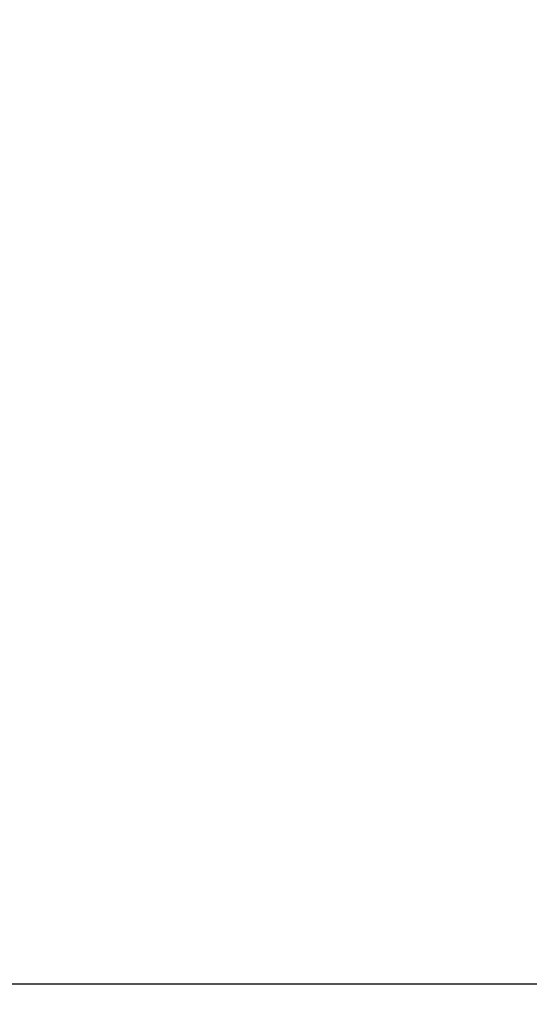
# Model space of a CAD drawing. Units: millimetres. Extents: x 0 to 2267, y 0 to 1823.
# Tile 7 of 256: x 1459 to 1482, y 1116 to 1162. Entities that reach past the tile are written whole.
import ezdxf

# ---------------------------------------------------------------- set-up
doc = ezdxf.new("R2010")
doc.units = ezdxf.units.MM
doc.header["$MEASUREMENT"] = 0
doc.layers.add('M-DIMS', color=2, linetype='Continuous', lineweight=25)
doc.layers.add('M-HATC', color=252, linetype='Continuous', lineweight=18)
doc.styles.get("Standard").update_dxf_attribs({"font": 'arial.ttf'})
doc.dimstyles.get("Standard").update_dxf_attribs({"dimtxt": 7, "dimasz": 4, "dimexe": 0.18, "dimexo": 0.0625, "dimgap": 0.09, "dimtad": 0, "dimdec": 0, "dimzin": 0, "dimdsep": 46, "dimtxsty": 'Standard', "dimcen": 0.09, "dimadec": 0, "dimazin": 0, "dimtfac": 1, "dimtdec": 0, "dimtofl": 0, "dimtmove": 0, "dimatfit": 3, "dimfxl": 1, "dimtolj": 1, "dimtzin": 0, "dimarcsym": 0})

# ---------------------------------------------------------------- blocks, each defined once
blk = doc.blocks.new('*D9')
at = {"layer": 'Defpoints', "color": 0, "transparency": 16777216}
for p in [(1332.087, 1117.417), (1505.929, 1117.417), (1505.929, 1077.417)]:
    blk.add_point(p, dxfattribs=at)
at = {"layer": 'M-DIMS', "color": 0, "lineweight": -2, "transparency": 16777216}
for p, q in [((1505.866, 1117.417), (1331.907, 1117.417)), ((1332.087, 1113.417), (1332.087, 1102.65)), ((1332.087, 1081.417), (1332.087, 1092.184)), ((1505.866, 1077.417), (1331.907, 1077.417))]:
    blk.add_line(p, q, dxfattribs=at)
at = {"layer": 'M-DIMS', "color": 0, "transparency": 16777216}
for points in [[(1331.42, 1113.417), (1332.753, 1113.417), (1332.087, 1117.417)], [(1331.42, 1081.417), (1332.753, 1081.417), (1332.087, 1077.417)]]:
    blk.add_solid(points, dxfattribs=at)
at = {"layer": 'M-DIMS', "color": 0, "transparency": 16777216, "insert": (1332.087, 1097.417), "char_height": 7, "attachment_point": 5, "rotation": 90}
blk.add_mtext('\\A1;40', dxfattribs=at)
blk = doc.blocks.new('*D10')
at = {"layer": 'Defpoints', "color": 0, "transparency": 16777216}
for p in [(1332.087, 1287.766), (1505.929, 1287.766), (1505.929, 1117.417)]:
    blk.add_point(p, dxfattribs=at)
at = {"layer": 'M-DIMS', "color": 0, "lineweight": -2, "transparency": 16777216}
for p, q in [((1505.866, 1287.766), (1331.907, 1287.766)), ((1332.087, 1283.766), (1332.087, 1216.908)), ((1332.087, 1121.417), (1332.087, 1188.275)), ((1505.866, 1117.417), (1331.907, 1117.417))]:
    blk.add_line(p, q, dxfattribs=at)
at = {"layer": 'M-DIMS', "color": 0, "transparency": 16777216}
for points in [[(1331.42, 1283.766), (1332.753, 1283.766), (1332.087, 1287.766)], [(1331.42, 1121.417), (1332.753, 1121.417), (1332.087, 1117.417)]]:
    blk.add_solid(points, dxfattribs=at)
at = {"layer": 'M-DIMS', "color": 0, "transparency": 16777216, "insert": (1332.087, 1202.591), "char_height": 7, "attachment_point": 5, "rotation": 90}
blk.add_mtext('\\A1;170.35', dxfattribs=at)

msp = doc.modelspace()

# ---------------------------------------------------------------- hatches: boundary and pattern name
at = {"layer": 'M-HATC'}
h = msp.add_hatch(color=256, dxfattribs=at)
h.dxf.hatch_style = 1
h.paths.add_polyline_path([(2055.771, 1603.062), (1381.087, 1603.062), (1381.087, 1598.062), (2055.771, 1598.062)])
h.paths.add_polyline_path([(2055.771, 1598.062), (1381.087, 1598.062), (1381.087, 1593.062), (2055.771, 1593.062)])
h.paths.add_polyline_path([(2051.307, 1536.761), (1385.55, 1536.761), (1385.55, 1526.761), (1387.55, 1526.761), (1388.537, 1525.053), (1385.332, 1521.233), (1385.332, 1521.223), (2050.254, 1522.749), (2048.321, 1525.053), (2049.307, 1526.761), (2051.307, 1526.761)])
edge = h.paths.add_edge_path()
edge.add_arc((1847.535, 1379.149), 135, 222.60306, 222.89085, ccw=False)
edge.add_line((1748.166, 1287.766), (1683.092, 1287.766))
edge.add_arc((1583.724, 1379.149), 135, 317.10915, 317.39694, ccw=False)
edge.add_arc((1678.969, 1290.671), 5, 222.8909, 317.1091, ccw=False)
edge.add_arc((1774.213, 1379.149), 135, 222.60306, 222.89085, ccw=False)
edge.add_line((1674.845, 1287.766), (1609.771, 1287.766))
edge.add_arc((1510.403, 1379.149), 135, 317.10915, 317.39694, ccw=False)
edge.add_arc((1605.647, 1290.671), 5, 222.8909, 317.1091, ccw=False)
edge.add_arc((1700.892, 1379.149), 135, 222.60306, 222.89085, ccw=False)
edge.add_line((1601.524, 1287.766), (1536.45, 1287.766))
edge.add_arc((1437.081, 1379.149), 135, 317.10915, 317.39694, ccw=False)
edge.add_arc((1532.326, 1290.671), 5, 222.8909, 317.1091, ccw=False)
edge.add_arc((1627.571, 1379.149), 135, 222.60306, 222.89085, ccw=False)
edge.add_line((1528.203, 1287.766), (1505.929, 1287.766))
edge.add_spline(control_points=[(1505.929, 1287.766), (1504.262, 1287.766), (1504.262, 1282.766), (1505.929, 1282.766)], knot_values=[0, 0, 0, 0, 5, 5, 5, 5], degree=3, periodic=0)
edge.add_line((1505.929, 1282.766), (1930.929, 1282.766))
edge.add_spline(control_points=[(1930.929, 1282.766), (1932.596, 1282.766), (1932.596, 1287.766), (1930.929, 1287.766)], knot_values=[0, 0, 0, 0, 5, 5, 5, 5], degree=3, periodic=0)
edge.add_line((1930.929, 1287.766), (1903.056, 1287.766))
edge.add_arc((1803.688, 1379.149), 135, 317.10915, 317.39694, ccw=False)
edge.add_arc((1898.932, 1290.671), 5, 222.8909, 317.1091, ccw=False)
edge.add_arc((1994.177, 1379.149), 135, 222.60306, 222.89085, ccw=False)
edge.add_line((1894.809, 1287.766), (1829.735, 1287.766))
edge.add_arc((1730.366, 1379.149), 135, 317.10915, 317.39694, ccw=False)
edge.add_arc((1825.611, 1290.671), 5, 222.8909, 317.1091, ccw=False)
edge.add_arc((1920.856, 1379.149), 135, 222.60306, 222.89085, ccw=False)
edge.add_line((1821.487, 1287.766), (1756.413, 1287.766))
edge.add_arc((1657.045, 1379.149), 135, 317.10915, 317.39694, ccw=False)
edge.add_arc((1752.29, 1290.671), 5, 222.8909, 317.1091, ccw=False)
edge = h.paths.add_edge_path()
edge.add_spline(control_points=[(1843.429, 1227.247), (1845.096, 1227.247), (1845.096, 1232.247), (1843.429, 1232.247)], knot_values=[0, 0, 0, 0, 5, 5, 5, 5], degree=3, periodic=0)
edge.add_line((1843.429, 1232.247), (1593.429, 1232.247))
edge.add_spline(control_points=[(1593.429, 1232.247), (1591.762, 1232.247), (1591.762, 1227.247), (1593.429, 1227.247)], knot_values=[0, 0, 0, 0, 5, 5, 5, 5], degree=3, periodic=0)
edge.add_line((1593.429, 1227.247), (1843.429, 1227.247))
h.paths.add_polyline_path([(1905.929, 1127.417), (1530.929, 1127.417, 0.414214), (1520.929, 1117.417), (1530.929, 1117.417), (1915.929, 1117.417, 0.414214)])
edge = h.paths.add_edge_path()
edge.add_arc((1397.086, 1498.408), 12.73, 90.7821, 190.8787, ccw=False)
edge.add_line((1396.912, 1511.136), (1428.01, 1511.349))
edge.add_line((1428.01, 1511.349), (1433.01, 1511.349))
edge.add_line((1433.01, 1511.349), (1434.439, 1511.349))
edge.add_arc((1419.474, 1498.08), 20, 41.561, 74.0821)
edge.add_line((1424.959, 1517.314), (1399.935, 1517.256))
edge.add_spline(control_points=[(1399.931, 1517.256), (1399.884, 1517.213), (1399.833, 1517.169), (1399.777, 1517.124)], knot_values=[11.567499, 11.567499, 11.567499, 11.567499, 11.814249, 11.814249, 11.814249, 11.814249], degree=3, periodic=0)
edge.add_spline(control_points=[(1399.633, 1517.01), (1399.583, 1516.972), (1399.531, 1516.934), (1399.476, 1516.895)], knot_values=[11.167718, 11.167718, 11.167718, 11.167718, 11.365188, 11.365188, 11.365188, 11.365188], degree=3, periodic=0)
edge.add_spline(control_points=[(1399.34, 1516.8), (1399.151, 1516.672), (1398.938, 1516.538), (1398.704, 1516.399)], knot_values=[10.376405, 10.376405, 10.376405, 10.376405, 11.00994, 11.00994, 11.00994, 11.00994], degree=3, periodic=0)
edge.add_spline(control_points=[(1398.657, 1516.372), (1398.579, 1516.326), (1398.498, 1516.28), (1398.415, 1516.233)], knot_values=[10.125175, 10.125175, 10.125175, 10.125175, 10.334406, 10.334406, 10.334406, 10.334406], degree=3, periodic=0)
edge.add_spline(control_points=[(1398.264, 1516.149), (1398.196, 1516.111), (1398.126, 1516.073), (1398.055, 1516.035)], knot_values=[9.832246, 9.832246, 9.832246, 9.832246, 9.999658, 9.999658, 9.999658, 9.999658], degree=3, periodic=0)
edge.add_spline(control_points=[(1397.999, 1516.005), (1397.731, 1515.862), (1397.446, 1515.717), (1397.147, 1515.571)], knot_values=[9.161808, 9.161808, 9.161808, 9.161808, 9.787769, 9.787769, 9.787769, 9.787769], degree=3, periodic=0)
edge.add_spline(control_points=[(1397.147, 1515.571), (1396.842, 1515.423), (1396.522, 1515.274), (1396.191, 1515.126)], knot_values=[8.524455, 8.524455, 8.524455, 8.524455, 9.161808, 9.161808, 9.161808, 9.161808], degree=3, periodic=0)
edge.add_spline(control_points=[(1396.078, 1515.076), (1395.985, 1515.035), (1395.892, 1514.994), (1395.798, 1514.953)], knot_values=[8.275193, 8.275193, 8.275193, 8.275193, 8.451726, 8.451726, 8.451726, 8.451726], degree=3, periodic=0)
edge.add_spline(control_points=[(1395.602, 1514.869), (1395.5, 1514.826), (1395.397, 1514.782), (1395.293, 1514.739)], knot_values=[7.962917, 7.962917, 7.962917, 7.962917, 8.152764, 8.152764, 8.152764, 8.152764], degree=3, periodic=0)
edge.add_spline(control_points=[(1395.212, 1514.706), (1394.828, 1514.547), (1394.435, 1514.393), (1394.036, 1514.244)], knot_values=[7.21254, 7.21254, 7.21254, 7.21254, 7.913148, 7.913148, 7.913148, 7.913148], degree=3, periodic=0)
edge.add_spline(control_points=[(1394.036, 1514.244), (1393.708, 1514.121), (1393.375, 1514.003), (1393.043, 1513.889)], knot_values=[6.633733, 6.633733, 6.633733, 6.633733, 7.21254, 7.21254, 7.21254, 7.21254], degree=3, periodic=0)
edge.add_spline(control_points=[(1392.821, 1513.815), (1392.72, 1513.781), (1392.618, 1513.748), (1392.517, 1513.715)], knot_values=[6.328796, 6.328796, 6.328796, 6.328796, 6.505493, 6.505493, 6.505493, 6.505493], degree=3, periodic=0)
edge.add_spline(control_points=[(1392.517, 1513.715), (1392.319, 1513.652), (1392.121, 1513.59), (1391.924, 1513.531)], knot_values=[5.984605, 5.984605, 5.984605, 5.984605, 6.328796, 6.328796, 6.328796, 6.328796], degree=3, periodic=0)
edge.add_spline(control_points=[(1391.792, 1513.491), (1391.312, 1513.35), (1390.838, 1513.224), (1390.378, 1513.117)], knot_values=[5.066697, 5.066697, 5.066697, 5.066697, 5.907055, 5.907055, 5.907055, 5.907055], degree=3, periodic=0)
edge.add_spline(control_points=[(1390.378, 1513.117), (1390.18, 1513.071), (1389.984, 1513.028), (1389.791, 1512.99)], knot_values=[4.70367, 4.70367, 4.70367, 4.70367, 5.066695, 5.066695, 5.066695, 5.066695], degree=3, periodic=0)
edge.add_spline(control_points=[(1389.422, 1512.92), (1389.246, 1512.889), (1389.073, 1512.862), (1388.904, 1512.838)], knot_values=[4.130571, 4.130571, 4.130571, 4.130571, 4.469816, 4.469816, 4.469816, 4.469816], degree=3, periodic=0)
edge.add_spline(control_points=[(1388.904, 1512.838), (1388.591, 1512.795), (1388.291, 1512.764), (1388.007, 1512.749)], knot_values=[3.504031, 3.504031, 3.504031, 3.504031, 4.130571, 4.130571, 4.130571, 4.130571], degree=3, periodic=0)
edge.add_spline(control_points=[(1387.936, 1512.746), (1387.854, 1512.742), (1387.773, 1512.74), (1387.694, 1512.739)], knot_values=[3.268866, 3.268866, 3.268866, 3.268866, 3.451164, 3.451164, 3.451164, 3.451164], degree=3, periodic=0)
edge.add_spline(control_points=[(1387.335, 1512.744), (1387.208, 1512.75), (1387.085, 1512.76), (1386.967, 1512.774)], knot_values=[2.670686, 2.670686, 2.670686, 2.670686, 2.984, 2.984, 2.984, 2.984], degree=3, periodic=0)
edge.add_spline(control_points=[(1386.833, 1512.792), (1386.821, 1512.794), (1386.809, 1512.796), (1386.797, 1512.798)], knot_values=[2.516981, 2.516981, 2.516981, 2.516981, 2.549528, 2.549528, 2.549528, 2.549528], degree=3, periodic=0)
edge.add_spline(control_points=[(1386.453, 1512.873), (1386.426, 1512.881), (1386.399, 1512.889), (1386.373, 1512.897)], knot_values=[2.095869, 2.095869, 2.095869, 2.095869, 2.17941, 2.17941, 2.17941, 2.17941], degree=3, periodic=0)
edge.add_spline(control_points=[(1386.069, 1513.019), (1386.063, 1513.022), (1386.058, 1513.025), (1386.052, 1513.028)], knot_values=[1.72453, 1.72453, 1.72453, 1.72453, 1.745933, 1.745933, 1.745933, 1.745933], degree=3, periodic=0)
edge.add_arc((1399.474, 1498.08), 20, 131.8243, 180)
edge.add_arc((1630.334, 1505.548), 250.971, 181.70518, 236.42798)
edge.add_arc((1605.34, 1483.304), 218.782, 238.66083, 243.34961)
edge.add_arc((1647.091, 1510.359), 262.899, 183.12984, 237.85344, ccw=False)
h.paths.add_polyline_path([(1406.537, 1391.964, 0.149382), (1491.551, 1296.442, -0.129517)], flags=17)
edge = h.paths.add_edge_path()
edge.add_arc((2037.384, 1498.08), 20, 0, 48.2659)
edge.add_spline(control_points=[(2050.697, 1513.005), (2050.651, 1512.985), (2050.603, 1512.966), (2050.554, 1512.948)], knot_values=[1.835652, 1.835652, 1.835652, 1.835652, 2.000781, 2.000781, 2.000781, 2.000781], degree=3, periodic=0)
edge.add_spline(control_points=[(2050.462, 1512.917), (2050.479, 1512.922), (2050.496, 1512.928), (2050.513, 1512.934)], knot_values=[2.045477, 2.045477, 2.045477, 2.045477, 2.101389, 2.101389, 2.101389, 2.101389], degree=3, periodic=0)
edge.add_spline(control_points=[(2050.129, 1512.834), (2050.198, 1512.847), (2050.266, 1512.862), (2050.331, 1512.879)], knot_values=[2.237629, 2.237629, 2.237629, 2.237629, 2.435841, 2.435841, 2.435841, 2.435841], degree=3, periodic=0)
edge.add_spline(control_points=[(2050.095, 1512.828), (2050.106, 1512.83), (2050.118, 1512.832), (2050.129, 1512.834)], knot_values=[2.435841, 2.435841, 2.435841, 2.435841, 2.468321, 2.468321, 2.468321, 2.468321], degree=3, periodic=0)
edge.add_spline(control_points=[(2049.784, 1512.785), (2049.855, 1512.792), (2049.924, 1512.801), (2049.992, 1512.811)], knot_values=[2.563852, 2.563852, 2.563852, 2.563852, 2.748541, 2.748541, 2.748541, 2.748541], degree=3, periodic=0)
edge.add_spline(control_points=[(2049.405, 1512.762), (2049.536, 1512.765), (2049.663, 1512.773), (2049.784, 1512.785)], knot_values=[2.748541, 2.748541, 2.748541, 2.748541, 3.064882, 3.064882, 3.064882, 3.064882], degree=3, periodic=0)
edge.add_spline(control_points=[(2049.17, 1512.76), (2049.234, 1512.759), (2049.297, 1512.759), (2049.358, 1512.761)], knot_values=[3.102309, 3.102309, 3.102309, 3.102309, 3.2503, 3.2503, 3.2503, 3.2503], degree=3, periodic=0)
edge.add_spline(control_points=[(2048.857, 1512.769), (2048.964, 1512.764), (2049.068, 1512.761), (2049.17, 1512.76)], knot_values=[3.2503, 3.2503, 3.2503, 3.2503, 3.486069, 3.486069, 3.486069, 3.486069], degree=3, periodic=0)
edge.add_spline(control_points=[(2048.692, 1512.779), (2048.373, 1512.801), (2048.035, 1512.841), (2047.682, 1512.897)], knot_values=[3.606429, 3.606429, 3.606429, 3.606429, 4.2989, 4.2989, 4.2989, 4.2989], degree=3, periodic=0)
edge.add_spline(control_points=[(2047.682, 1512.897), (2047.546, 1512.919), (2047.408, 1512.942), (2047.268, 1512.969)], knot_values=[4.2989, 4.2989, 4.2989, 4.2989, 4.565769, 4.565769, 4.565769, 4.565769], degree=3, periodic=0)
edge.add_spline(control_points=[(2047.268, 1512.969), (2047.145, 1512.991), (2047.021, 1513.016), (2046.895, 1513.042)], knot_values=[4.565769, 4.565769, 4.565769, 4.565769, 4.799971, 4.799971, 4.799971, 4.799971], degree=3, periodic=0)
edge.add_spline(control_points=[(2046.895, 1513.042), (2046.529, 1513.119), (2046.151, 1513.209), (2045.768, 1513.311)], knot_values=[4.799971, 4.799971, 4.799971, 4.799971, 5.483718, 5.483718, 5.483718, 5.483718], degree=3, periodic=0)
edge.add_spline(control_points=[(2045.768, 1513.311), (2045.372, 1513.415), (2044.97, 1513.532), (2044.566, 1513.659)], knot_values=[5.483718, 5.483718, 5.483718, 5.483718, 6.187866, 6.187866, 6.187866, 6.187866], degree=3, periodic=0)
edge.add_spline(control_points=[(2044.566, 1513.659), (2044.415, 1513.706), (2044.263, 1513.755), (2044.112, 1513.805)], knot_values=[6.187866, 6.187866, 6.187866, 6.187866, 6.451551, 6.451551, 6.451551, 6.451551], degree=3, periodic=0)
edge.add_spline(control_points=[(2044.112, 1513.805), (2043.997, 1513.843), (2043.882, 1513.881), (2043.767, 1513.92)], knot_values=[6.451551, 6.451551, 6.451551, 6.451551, 6.651434, 6.651434, 6.651434, 6.651434], degree=3, periodic=0)
edge.add_spline(control_points=[(2043.767, 1513.92), (2043.372, 1514.055), (2042.977, 1514.198), (2042.589, 1514.346)], knot_values=[6.651434, 6.651434, 6.651434, 6.651434, 7.338879, 7.338879, 7.338879, 7.338879], degree=3, periodic=0)
edge.add_spline(control_points=[(2042.589, 1514.346), (2042.164, 1514.507), (2041.746, 1514.675), (2041.341, 1514.846)], knot_values=[7.338879, 7.338879, 7.338879, 7.338879, 8.089209, 8.089209, 8.089209, 8.089209], degree=3, periodic=0)
edge.add_spline(control_points=[(2041.341, 1514.846), (2041.103, 1514.946), (2040.869, 1515.048), (2040.64, 1515.15)], knot_values=[8.089209, 8.089209, 8.089209, 8.089209, 8.529587, 8.529587, 8.529587, 8.529587], degree=3, periodic=0)
edge.add_spline(control_points=[(2040.51, 1515.209), (2040.082, 1515.402), (2039.675, 1515.597), (2039.295, 1515.789)], knot_values=[8.613818, 8.613818, 8.613818, 8.613818, 9.44571, 9.44571, 9.44571, 9.44571], degree=3, periodic=0)
edge.add_spline(control_points=[(2039.295, 1515.789), (2039.062, 1515.907), (2038.839, 1516.025), (2038.629, 1516.14)], knot_values=[9.44571, 9.44571, 9.44571, 9.44571, 9.956404, 9.956404, 9.956404, 9.956404], degree=3, periodic=0)
edge.add_spline(control_points=[(2038.629, 1516.14), (2038.519, 1516.2), (2038.412, 1516.26), (2038.309, 1516.319)], knot_values=[9.956404, 9.956404, 9.956404, 9.956404, 10.223542, 10.223542, 10.223542, 10.223542], degree=3, periodic=0)
edge.add_spline(control_points=[(2038.309, 1516.319), (2038.214, 1516.374), (2038.122, 1516.428), (2038.033, 1516.481)], knot_values=[10.223542, 10.223542, 10.223542, 10.223542, 10.47051, 10.47051, 10.47051, 10.47051], degree=3, periodic=0)
edge.add_spline(control_points=[(2038.033, 1516.481), (2037.786, 1516.63), (2037.564, 1516.773), (2037.372, 1516.909)], knot_values=[10.47051, 10.47051, 10.47051, 10.47051, 11.15767, 11.15767, 11.15767, 11.15767], degree=3, periodic=0)
edge.add_spline(control_points=[(2037.372, 1516.909), (2037.279, 1516.975), (2037.193, 1517.04), (2037.114, 1517.102)], knot_values=[11.15767, 11.15767, 11.15767, 11.15767, 11.49227, 11.49227, 11.49227, 11.49227], degree=3, periodic=0)
edge.add_spline(control_points=[(2036.856, 1517.326), (2036.915, 1517.269), (2036.981, 1517.21), (2037.056, 1517.149)], knot_values=[11.577341, 11.577341, 11.577341, 11.577341, 11.91035, 11.91035, 11.91035, 11.91035], degree=3, periodic=0)
edge.add_spline(control_points=[(2036.807, 1517.375), (2036.823, 1517.359), (2036.839, 1517.342), (2036.856, 1517.326)], knot_values=[11.91035, 11.91035, 11.91035, 11.91035, 12.007402, 12.007402, 12.007402, 12.007402], degree=3, periodic=0)
edge.add_spline(control_points=[(2036.702, 1517.494), (2036.71, 1517.483), (2036.72, 1517.472), (2036.729, 1517.461)], knot_values=[12.184155, 12.184155, 12.184155, 12.184155, 12.255409, 12.255409, 12.255409, 12.255409], degree=3, periodic=0)
edge.add_spline(control_points=[(2036.616, 1517.621), (2036.62, 1517.613), (2036.624, 1517.606), (2036.629, 1517.598)], knot_values=[12.487913, 12.487913, 12.487913, 12.487913, 12.541035, 12.541035, 12.541035, 12.541035], degree=3, periodic=0)
edge.add_spline(control_points=[(2036.563, 1517.786), (2036.564, 1517.779), (2036.564, 1517.773), (2036.565, 1517.766)], knot_values=[12.911761, 12.911761, 12.911761, 12.911761, 12.968286, 12.968286, 12.968286, 12.968286], degree=3, periodic=0)
edge.add_spline(control_points=[(2036.617, 1517.93), (2036.612, 1517.926), (2036.609, 1517.921), (2036.605, 1517.916)], knot_values=[13.382527, 13.382527, 13.382527, 13.382527, 13.433791, 13.433791, 13.433791, 13.433791], degree=3, periodic=0)
edge.add_spline(control_points=[(2036.749, 1518.017), (2036.736, 1518.012), (2036.724, 1518.006), (2036.712, 1518)], knot_values=[13.726299, 13.726299, 13.726299, 13.726299, 13.809928, 13.809928, 13.809928, 13.809928], degree=3, periodic=0)
edge.add_spline(control_points=[(2036.86, 1518.053), (2036.839, 1518.047), (2036.818, 1518.042), (2036.799, 1518.035)], knot_values=[13.910887, 13.910887, 13.910887, 13.910887, 14.02153, 14.02153, 14.02153, 14.02153], degree=3, periodic=0)
edge.add_line((2036.964, 1518.08), (2032.384, 1518.08))
edge.add_line((2032.384, 1518.08), (2027.384, 1518.08))
edge.add_line((2027.384, 1518.08), (2022.384, 1518.08))
edge.add_line((2022.384, 1518.08), (2017.384, 1518.08))
edge.add_arc((2017.384, 1498.08), 20, 90, 138.439)
edge.add_line((2002.419, 1511.349), (2003.848, 1511.349))
edge.add_line((2003.848, 1511.349), (2008.848, 1511.349))
edge.add_line((2008.848, 1511.349), (2039.772, 1511.138))
edge.add_arc((2039.772, 1498.408), 12.73, -10.8787, 90, ccw=False)
edge.add_arc((1789.767, 1510.359), 262.899, 302.14656, 356.87016, ccw=False)
edge.add_arc((1831.518, 1483.304), 218.782, 296.65039, 301.33917)
edge.add_arc((1806.524, 1505.548), 250.971, 303.57202, 358.29482)
h.paths.add_polyline_path([(2030.321, 1391.964, -0.129517), (1945.307, 1296.442, 0.149382)], flags=17)
edge = h.paths.add_edge_path()
edge.add_spline(control_points=[(2037.246, 1518.082), (2037.29, 1518.081), (2037.336, 1518.08), (2037.384, 1518.08)], knot_values=[0.000012, 0.000012, 0.000012, 0.000012, 0.144754, 0.144754, 0.144754, 0.144754], degree=3, periodic=0)
edge.add_line((2037.336, 1518.08), (2037.01, 1518.08))
edge.add_spline(control_points=[(2037.01, 1518.08), (2036.982, 1518.077), (2036.956, 1518.073), (2036.931, 1518.068)], knot_values=[14.13465, 14.13465, 14.13465, 14.13465, 14.247197, 14.247197, 14.247197, 14.247197], degree=3, periodic=0)
edge.add_spline(control_points=[(2036.931, 1518.068), (2036.928, 1518.067), (2036.924, 1518.067), (2036.921, 1518.066)], knot_values=[14.118315, 14.118315, 14.118315, 14.118315, 14.13465, 14.13465, 14.13465, 14.13465], degree=3, periodic=0)
edge.add_spline(control_points=[(2036.921, 1518.066), (2036.912, 1518.064), (2036.903, 1518.063), (2036.895, 1518.061)], knot_values=[14.078086, 14.078086, 14.078086, 14.078086, 14.118315, 14.118315, 14.118315, 14.118315], degree=3, periodic=0)
edge.add_spline(control_points=[(2036.895, 1518.061), (2036.883, 1518.058), (2036.872, 1518.056), (2036.86, 1518.053)], knot_values=[14.02153, 14.02153, 14.02153, 14.02153, 14.078086, 14.078086, 14.078086, 14.078086], degree=3, periodic=0)
edge.add_spline(control_points=[(2036.86, 1518.053), (2036.839, 1518.047), (2036.818, 1518.042), (2036.799, 1518.035)], knot_values=[13.910887, 13.910887, 13.910887, 13.910887, 14.02153, 14.02153, 14.02153, 14.02153], degree=3, periodic=0)
edge.add_spline(control_points=[(2036.799, 1518.035), (2036.798, 1518.035), (2036.797, 1518.035), (2036.797, 1518.035)], knot_values=[13.906906, 13.906906, 13.906906, 13.906906, 13.910887, 13.910887, 13.910887, 13.910887], degree=3, periodic=0)
edge.add_spline(control_points=[(2036.797, 1518.035), (2036.788, 1518.032), (2036.78, 1518.029), (2036.772, 1518.026)], knot_values=[13.857826, 13.857826, 13.857826, 13.857826, 13.906906, 13.906906, 13.906906, 13.906906], degree=3, periodic=0)
edge.add_spline(control_points=[(2036.772, 1518.026), (2036.764, 1518.023), (2036.756, 1518.02), (2036.749, 1518.017)], knot_values=[13.809928, 13.809928, 13.809928, 13.809928, 13.857826, 13.857826, 13.857826, 13.857826], degree=3, periodic=0)
edge.add_spline(control_points=[(2036.749, 1518.017), (2036.736, 1518.012), (2036.724, 1518.006), (2036.712, 1518)], knot_values=[13.726299, 13.726299, 13.726299, 13.726299, 13.809928, 13.809928, 13.809928, 13.809928], degree=3, periodic=0)
edge.add_spline(control_points=[(2036.712, 1518), (2036.712, 1518), (2036.712, 1518), (2036.711, 1518)], knot_values=[13.723993, 13.723993, 13.723993, 13.723993, 13.726299, 13.726299, 13.726299, 13.726299], degree=3, periodic=0)
edge.add_spline(control_points=[(2036.711, 1518), (2036.706, 1517.997), (2036.701, 1517.994), (2036.696, 1517.992)], knot_values=[13.686536, 13.686536, 13.686536, 13.686536, 13.723993, 13.723993, 13.723993, 13.723993], degree=3, periodic=0)
edge.add_spline(control_points=[(2036.696, 1517.992), (2036.692, 1517.989), (2036.687, 1517.987), (2036.683, 1517.984)], knot_values=[13.651251, 13.651251, 13.651251, 13.651251, 13.686536, 13.686536, 13.686536, 13.686536], degree=3, periodic=0)
edge.add_spline(control_points=[(2036.683, 1517.984), (2036.676, 1517.98), (2036.67, 1517.976), (2036.664, 1517.971)], knot_values=[13.596804, 13.596804, 13.596804, 13.596804, 13.651251, 13.651251, 13.651251, 13.651251], degree=3, periodic=0)
edge.add_spline(control_points=[(2036.664, 1517.971), (2036.664, 1517.971), (2036.663, 1517.971), (2036.663, 1517.971)], knot_values=[13.593956, 13.593956, 13.593956, 13.593956, 13.596804, 13.596804, 13.596804, 13.596804], degree=3, periodic=0)
edge.add_spline(control_points=[(2036.663, 1517.971), (2036.66, 1517.969), (2036.658, 1517.967), (2036.655, 1517.965)], knot_values=[13.570322, 13.570322, 13.570322, 13.570322, 13.593956, 13.593956, 13.593956, 13.593956], degree=3, periodic=0)
edge.add_spline(control_points=[(2036.655, 1517.965), (2036.653, 1517.963), (2036.65, 1517.961), (2036.647, 1517.959)], knot_values=[13.545477, 13.545477, 13.545477, 13.545477, 13.570322, 13.570322, 13.570322, 13.570322], degree=3, periodic=0)
edge.add_spline(control_points=[(2036.647, 1517.959), (2036.647, 1517.959), (2036.647, 1517.959), (2036.647, 1517.959)], knot_values=[13.543931, 13.543931, 13.543931, 13.543931, 13.545477, 13.545477, 13.545477, 13.545477], degree=3, periodic=0)
edge.add_spline(control_points=[(2036.647, 1517.959), (2036.641, 1517.954), (2036.636, 1517.949), (2036.631, 1517.945)], knot_values=[13.488237, 13.488237, 13.488237, 13.488237, 13.543931, 13.543931, 13.543931, 13.543931], degree=3, periodic=0)
edge.add_spline(control_points=[(2036.631, 1517.945), (2036.628, 1517.942), (2036.626, 1517.94), (2036.623, 1517.937)], knot_values=[13.460307, 13.460307, 13.460307, 13.460307, 13.488237, 13.488237, 13.488237, 13.488237], degree=3, periodic=0)
edge.add_spline(control_points=[(2036.623, 1517.937), (2036.622, 1517.936), (2036.62, 1517.934), (2036.618, 1517.932)], knot_values=[13.439712, 13.439712, 13.439712, 13.439712, 13.460307, 13.460307, 13.460307, 13.460307], degree=3, periodic=0)
edge.add_spline(control_points=[(2036.618, 1517.932), (2036.618, 1517.931), (2036.617, 1517.931), (2036.617, 1517.93)], knot_values=[13.433791, 13.433791, 13.433791, 13.433791, 13.439712, 13.439712, 13.439712, 13.439712], degree=3, periodic=0)
edge.add_spline(control_points=[(2036.617, 1517.93), (2036.612, 1517.926), (2036.609, 1517.921), (2036.605, 1517.916)], knot_values=[13.382527, 13.382527, 13.382527, 13.382527, 13.433791, 13.433791, 13.433791, 13.433791], degree=3, periodic=0)
edge.add_spline(control_points=[(2036.605, 1517.916), (2036.603, 1517.913), (2036.6, 1517.91), (2036.598, 1517.907)], knot_values=[13.350017, 13.350017, 13.350017, 13.350017, 13.382527, 13.382527, 13.382527, 13.382527], degree=3, periodic=0)
edge.add_spline(control_points=[(2036.598, 1517.907), (2036.597, 1517.906), (2036.596, 1517.904), (2036.595, 1517.903)], knot_values=[13.333922, 13.333922, 13.333922, 13.333922, 13.350017, 13.350017, 13.350017, 13.350017], degree=3, periodic=0)
edge.add_spline(control_points=[(2036.595, 1517.903), (2036.595, 1517.902), (2036.594, 1517.901), (2036.593, 1517.9)], knot_values=[13.323828, 13.323828, 13.323828, 13.323828, 13.333922, 13.333922, 13.333922, 13.333922], degree=3, periodic=0)
edge.add_spline(control_points=[(2036.593, 1517.9), (2036.59, 1517.895), (2036.588, 1517.891), (2036.585, 1517.886)], knot_values=[13.277545, 13.277545, 13.277545, 13.277545, 13.323828, 13.323828, 13.323828, 13.323828], degree=3, periodic=0)
edge.add_spline(control_points=[(2036.585, 1517.886), (2036.584, 1517.883), (2036.582, 1517.879), (2036.58, 1517.875)], knot_values=[13.240119, 13.240119, 13.240119, 13.240119, 13.277545, 13.277545, 13.277545, 13.277545], degree=3, periodic=0)
edge.add_spline(control_points=[(2036.58, 1517.875), (2036.58, 1517.874), (2036.579, 1517.873), (2036.578, 1517.872)], knot_values=[13.228211, 13.228211, 13.228211, 13.228211, 13.240119, 13.240119, 13.240119, 13.240119], degree=3, periodic=0)
edge.add_spline(control_points=[(2036.578, 1517.872), (2036.578, 1517.87), (2036.577, 1517.869), (2036.577, 1517.868)], knot_values=[13.215717, 13.215717, 13.215717, 13.215717, 13.228211, 13.228211, 13.228211, 13.228211], degree=3, periodic=0)
edge.add_spline(control_points=[(2036.577, 1517.868), (2036.575, 1517.864), (2036.574, 1517.86), (2036.573, 1517.857)], knot_values=[13.179847, 13.179847, 13.179847, 13.179847, 13.215717, 13.215717, 13.215717, 13.215717], degree=3, periodic=0)
edge.add_spline(control_points=[(2036.573, 1517.857), (2036.571, 1517.851), (2036.57, 1517.846), (2036.569, 1517.841)], knot_values=[13.132017, 13.132017, 13.132017, 13.132017, 13.179847, 13.179847, 13.179847, 13.179847], degree=3, periodic=0)
edge.add_spline(control_points=[(2036.569, 1517.841), (2036.568, 1517.84), (2036.568, 1517.839), (2036.568, 1517.838)], knot_values=[13.122482, 13.122482, 13.122482, 13.122482, 13.132017, 13.132017, 13.132017, 13.132017], degree=3, periodic=0)
edge.add_spline(control_points=[(2036.568, 1517.838), (2036.568, 1517.836), (2036.567, 1517.835), (2036.567, 1517.833)], knot_values=[13.105592, 13.105592, 13.105592, 13.105592, 13.122482, 13.122482, 13.122482, 13.122482], degree=3, periodic=0)
edge.add_spline(control_points=[(2036.567, 1517.833), (2036.566, 1517.829), (2036.566, 1517.826), (2036.565, 1517.822)], knot_values=[13.074063, 13.074063, 13.074063, 13.074063, 13.105592, 13.105592, 13.105592, 13.105592], degree=3, periodic=0)
edge.add_spline(control_points=[(2036.565, 1517.822), (2036.565, 1517.822), (2036.565, 1517.822), (2036.565, 1517.822)], knot_values=[13.074043, 13.074043, 13.074043, 13.074043, 13.074063, 13.074063, 13.074063, 13.074063], degree=3, periodic=0)
edge.add_spline(control_points=[(2036.565, 1517.822), (2036.564, 1517.816), (2036.564, 1517.811), (2036.564, 1517.805)], knot_values=[13.021884, 13.021884, 13.021884, 13.021884, 13.074043, 13.074043, 13.074043, 13.074043], degree=3, periodic=0)
edge.add_spline(control_points=[(2036.564, 1517.805), (2036.564, 1517.804), (2036.564, 1517.803), (2036.564, 1517.803)], knot_values=[13.01674, 13.01674, 13.01674, 13.01674, 13.021884, 13.021884, 13.021884, 13.021884], degree=3, periodic=0)
edge.add_spline(control_points=[(2036.564, 1517.803), (2036.563, 1517.801), (2036.563, 1517.798), (2036.563, 1517.796)], knot_values=[12.996438, 12.996438, 12.996438, 12.996438, 13.01674, 13.01674, 13.01674, 13.01674], degree=3, periodic=0)
edge.add_spline(control_points=[(2036.563, 1517.796), (2036.563, 1517.793), (2036.563, 1517.789), (2036.563, 1517.786)], knot_values=[12.968286, 12.968286, 12.968286, 12.968286, 12.996438, 12.996438, 12.996438, 12.996438], degree=3, periodic=0)
edge.add_spline(control_points=[(2036.563, 1517.786), (2036.564, 1517.779), (2036.564, 1517.773), (2036.565, 1517.766)], knot_values=[12.911761, 12.911761, 12.911761, 12.911761, 12.968286, 12.968286, 12.968286, 12.968286], degree=3, periodic=0)
edge.add_spline(control_points=[(2036.565, 1517.766), (2036.565, 1517.766), (2036.565, 1517.766), (2036.565, 1517.766)], knot_values=[12.911017, 12.911017, 12.911017, 12.911017, 12.911761, 12.911761, 12.911761, 12.911761], degree=3, periodic=0)
edge.add_spline(control_points=[(2036.565, 1517.766), (2036.565, 1517.762), (2036.566, 1517.759), (2036.566, 1517.756)], knot_values=[12.88528, 12.88528, 12.88528, 12.88528, 12.911017, 12.911017, 12.911017, 12.911017], degree=3, periodic=0)
edge.add_spline(control_points=[(2036.566, 1517.756), (2036.567, 1517.753), (2036.567, 1517.751), (2036.568, 1517.748)], knot_values=[12.862519, 12.862519, 12.862519, 12.862519, 12.88528, 12.88528, 12.88528, 12.88528], degree=3, periodic=0)
edge.add_spline(control_points=[(2036.568, 1517.748), (2036.568, 1517.747), (2036.568, 1517.747), (2036.568, 1517.746)], knot_values=[12.858885, 12.858885, 12.858885, 12.858885, 12.862519, 12.862519, 12.862519, 12.862519], degree=3, periodic=0)
edge.add_spline(control_points=[(2036.568, 1517.746), (2036.569, 1517.74), (2036.571, 1517.733), (2036.572, 1517.726)], knot_values=[12.8053, 12.8053, 12.8053, 12.8053, 12.858885, 12.858885, 12.858885, 12.858885], degree=3, periodic=0)
edge.add_spline(control_points=[(2036.572, 1517.726), (2036.573, 1517.723), (2036.574, 1517.719), (2036.576, 1517.715)], knot_values=[12.775176, 12.775176, 12.775176, 12.775176, 12.8053, 12.8053, 12.8053, 12.8053], degree=3, periodic=0)
edge.add_spline(control_points=[(2036.576, 1517.715), (2036.576, 1517.713), (2036.577, 1517.71), (2036.578, 1517.708)], knot_values=[12.756759, 12.756759, 12.756759, 12.756759, 12.775176, 12.775176, 12.775176, 12.775176], degree=3, periodic=0)
edge.add_spline(control_points=[(2036.578, 1517.708), (2036.578, 1517.707), (2036.578, 1517.706), (2036.579, 1517.705)], knot_values=[12.748742, 12.748742, 12.748742, 12.748742, 12.756759, 12.756759, 12.756759, 12.756759], degree=3, periodic=0)
edge.add_spline(control_points=[(2036.579, 1517.705), (2036.581, 1517.698), (2036.583, 1517.692), (2036.586, 1517.685)], knot_values=[12.69959, 12.69959, 12.69959, 12.69959, 12.748742, 12.748742, 12.748742, 12.748742], degree=3, periodic=0)
edge.add_spline(control_points=[(2036.586, 1517.685), (2036.588, 1517.68), (2036.59, 1517.675), (2036.592, 1517.669)], knot_values=[12.659038, 12.659038, 12.659038, 12.659038, 12.69959, 12.69959, 12.69959, 12.69959], degree=3, periodic=0)
edge.add_spline(control_points=[(2036.592, 1517.669), (2036.594, 1517.665), (2036.596, 1517.66), (2036.598, 1517.656)], knot_values=[12.626806, 12.626806, 12.626806, 12.626806, 12.659038, 12.659038, 12.659038, 12.659038], degree=3, periodic=0)
edge.add_spline(control_points=[(2036.598, 1517.656), (2036.598, 1517.655), (2036.599, 1517.654), (2036.599, 1517.653)], knot_values=[12.619394, 12.619394, 12.619394, 12.619394, 12.626806, 12.626806, 12.626806, 12.626806], degree=3, periodic=0)
edge.add_spline(control_points=[(2036.599, 1517.653), (2036.604, 1517.642), (2036.61, 1517.632), (2036.616, 1517.621)], knot_values=[12.541039, 12.541039, 12.541039, 12.541039, 12.619394, 12.619394, 12.619394, 12.619394], degree=3, periodic=0)
edge.add_spline(control_points=[(2036.616, 1517.621), (2036.616, 1517.621), (2036.616, 1517.621), (2036.616, 1517.621)], knot_values=[12.541035, 12.541035, 12.541035, 12.541035, 12.541039, 12.541039, 12.541039, 12.541039], degree=3, periodic=0)
edge.add_spline(control_points=[(2036.616, 1517.621), (2036.62, 1517.613), (2036.624, 1517.606), (2036.629, 1517.598)], knot_values=[12.487913, 12.487913, 12.487913, 12.487913, 12.541035, 12.541035, 12.541035, 12.541035], degree=3, periodic=0)
edge.add_spline(control_points=[(2036.629, 1517.598), (2036.633, 1517.592), (2036.637, 1517.585), (2036.641, 1517.579)], knot_values=[12.443982, 12.443982, 12.443982, 12.443982, 12.487913, 12.487913, 12.487913, 12.487913], degree=3, periodic=0)
edge.add_spline(control_points=[(2036.641, 1517.579), (2036.641, 1517.578), (2036.642, 1517.576), (2036.643, 1517.575)], knot_values=[12.434996, 12.434996, 12.434996, 12.434996, 12.443982, 12.443982, 12.443982, 12.443982], degree=3, periodic=0)
edge.add_spline(control_points=[(2036.643, 1517.575), (2036.653, 1517.56), (2036.664, 1517.544), (2036.676, 1517.528)], knot_values=[12.329647, 12.329647, 12.329647, 12.329647, 12.434996, 12.434996, 12.434996, 12.434996], degree=3, periodic=0)
edge.add_spline(control_points=[(2036.676, 1517.528), (2036.684, 1517.517), (2036.693, 1517.505), (2036.702, 1517.494)], knot_values=[12.255409, 12.255409, 12.255409, 12.255409, 12.329647, 12.329647, 12.329647, 12.329647], degree=3, periodic=0)
edge.add_spline(control_points=[(2036.702, 1517.494), (2036.71, 1517.483), (2036.72, 1517.472), (2036.729, 1517.461)], knot_values=[12.184155, 12.184155, 12.184155, 12.184155, 12.255409, 12.255409, 12.255409, 12.255409], degree=3, periodic=0)
edge.add_spline(control_points=[(2036.729, 1517.461), (2036.744, 1517.444), (2036.759, 1517.426), (2036.775, 1517.409)], knot_values=[12.075961, 12.075961, 12.075961, 12.075961, 12.184155, 12.184155, 12.184155, 12.184155], degree=3, periodic=0)
edge.add_spline(control_points=[(2036.775, 1517.409), (2036.776, 1517.407), (2036.777, 1517.406), (2036.778, 1517.405)], knot_values=[12.069502, 12.069502, 12.069502, 12.069502, 12.075961, 12.075961, 12.075961, 12.075961], degree=3, periodic=0)
edge.add_spline(control_points=[(2036.778, 1517.405), (2036.788, 1517.395), (2036.797, 1517.385), (2036.807, 1517.375)], knot_values=[12.007402, 12.007402, 12.007402, 12.007402, 12.069502, 12.069502, 12.069502, 12.069502], degree=3, periodic=0)
edge.add_spline(control_points=[(2036.807, 1517.375), (2036.823, 1517.359), (2036.839, 1517.342), (2036.856, 1517.326)], knot_values=[11.91035, 11.91035, 11.91035, 11.91035, 12.007402, 12.007402, 12.007402, 12.007402], degree=3, periodic=0)
edge.add_spline(control_points=[(2036.856, 1517.326), (2036.915, 1517.269), (2036.981, 1517.21), (2037.056, 1517.149)], knot_values=[11.577341, 11.577341, 11.577341, 11.577341, 11.91035, 11.91035, 11.91035, 11.91035], degree=3, periodic=0)
edge.add_spline(control_points=[(2037.056, 1517.149), (2037.075, 1517.134), (2037.094, 1517.118), (2037.114, 1517.102)], knot_values=[11.49227, 11.49227, 11.49227, 11.49227, 11.577341, 11.577341, 11.577341, 11.577341], degree=3, periodic=0)
edge.add_spline(control_points=[(2037.114, 1517.102), (2037.193, 1517.04), (2037.279, 1516.975), (2037.372, 1516.909)], knot_values=[11.15767, 11.15767, 11.15767, 11.15767, 11.49227, 11.49227, 11.49227, 11.49227], degree=3, periodic=0)
edge.add_spline(control_points=[(2037.372, 1516.909), (2037.564, 1516.773), (2037.786, 1516.63), (2038.033, 1516.481)], knot_values=[10.47051, 10.47051, 10.47051, 10.47051, 11.15767, 11.15767, 11.15767, 11.15767], degree=3, periodic=0)
edge.add_spline(control_points=[(2038.033, 1516.481), (2038.122, 1516.428), (2038.214, 1516.374), (2038.309, 1516.319)], knot_values=[10.223542, 10.223542, 10.223542, 10.223542, 10.47051, 10.47051, 10.47051, 10.47051], degree=3, periodic=0)
edge.add_spline(control_points=[(2038.309, 1516.319), (2038.412, 1516.26), (2038.519, 1516.2), (2038.629, 1516.14)], knot_values=[9.956404, 9.956404, 9.956404, 9.956404, 10.223542, 10.223542, 10.223542, 10.223542], degree=3, periodic=0)
edge.add_spline(control_points=[(2038.629, 1516.14), (2038.839, 1516.025), (2039.062, 1515.907), (2039.295, 1515.789)], knot_values=[9.44571, 9.44571, 9.44571, 9.44571, 9.956404, 9.956404, 9.956404, 9.956404], degree=3, periodic=0)
edge.add_spline(control_points=[(2039.295, 1515.789), (2039.675, 1515.597), (2040.082, 1515.402), (2040.51, 1515.209)], knot_values=[8.613818, 8.613818, 8.613818, 8.613818, 9.44571, 9.44571, 9.44571, 9.44571], degree=3, periodic=0)
edge.add_spline(control_points=[(2040.51, 1515.209), (2040.553, 1515.189), (2040.597, 1515.17), (2040.64, 1515.15)], knot_values=[8.529587, 8.529587, 8.529587, 8.529587, 8.613818, 8.613818, 8.613818, 8.613818], degree=3, periodic=0)
edge.add_spline(control_points=[(2040.64, 1515.15), (2040.869, 1515.048), (2041.103, 1514.946), (2041.341, 1514.846)], knot_values=[8.089209, 8.089209, 8.089209, 8.089209, 8.529587, 8.529587, 8.529587, 8.529587], degree=3, periodic=0)
edge.add_spline(control_points=[(2041.341, 1514.846), (2041.746, 1514.675), (2042.164, 1514.507), (2042.589, 1514.346)], knot_values=[7.338879, 7.338879, 7.338879, 7.338879, 8.089209, 8.089209, 8.089209, 8.089209], degree=3, periodic=0)
edge.add_spline(control_points=[(2042.589, 1514.346), (2042.977, 1514.198), (2043.372, 1514.055), (2043.767, 1513.92)], knot_values=[6.651434, 6.651434, 6.651434, 6.651434, 7.338879, 7.338879, 7.338879, 7.338879], degree=3, periodic=0)
edge.add_spline(control_points=[(2043.767, 1513.92), (2043.882, 1513.881), (2043.997, 1513.843), (2044.112, 1513.805)], knot_values=[6.451551, 6.451551, 6.451551, 6.451551, 6.651434, 6.651434, 6.651434, 6.651434], degree=3, periodic=0)
edge.add_spline(control_points=[(2044.112, 1513.805), (2044.263, 1513.755), (2044.415, 1513.706), (2044.566, 1513.659)], knot_values=[6.187866, 6.187866, 6.187866, 6.187866, 6.451551, 6.451551, 6.451551, 6.451551], degree=3, periodic=0)
edge.add_spline(control_points=[(2044.566, 1513.659), (2044.97, 1513.532), (2045.372, 1513.415), (2045.768, 1513.311)], knot_values=[5.483718, 5.483718, 5.483718, 5.483718, 6.187866, 6.187866, 6.187866, 6.187866], degree=3, periodic=0)
edge.add_spline(control_points=[(2045.768, 1513.311), (2046.151, 1513.209), (2046.529, 1513.119), (2046.895, 1513.042)], knot_values=[4.799971, 4.799971, 4.799971, 4.799971, 5.483718, 5.483718, 5.483718, 5.483718], degree=3, periodic=0)
edge.add_spline(control_points=[(2046.895, 1513.042), (2047.021, 1513.016), (2047.145, 1512.991), (2047.268, 1512.969)], knot_values=[4.565769, 4.565769, 4.565769, 4.565769, 4.799971, 4.799971, 4.799971, 4.799971], degree=3, periodic=0)
edge.add_spline(control_points=[(2047.268, 1512.969), (2047.408, 1512.942), (2047.546, 1512.919), (2047.682, 1512.897)], knot_values=[4.2989, 4.2989, 4.2989, 4.2989, 4.565769, 4.565769, 4.565769, 4.565769], degree=3, periodic=0)
edge.add_spline(control_points=[(2047.682, 1512.897), (2048.035, 1512.841), (2048.373, 1512.801), (2048.692, 1512.779)], knot_values=[3.606429, 3.606429, 3.606429, 3.606429, 4.2989, 4.2989, 4.2989, 4.2989], degree=3, periodic=0)
edge.add_spline(control_points=[(2048.692, 1512.779), (2048.748, 1512.775), (2048.803, 1512.772), (2048.857, 1512.769)], knot_values=[3.486069, 3.486069, 3.486069, 3.486069, 3.606429, 3.606429, 3.606429, 3.606429], degree=3, periodic=0)
edge.add_spline(control_points=[(2048.857, 1512.769), (2048.964, 1512.764), (2049.068, 1512.761), (2049.17, 1512.76)], knot_values=[3.2503, 3.2503, 3.2503, 3.2503, 3.486069, 3.486069, 3.486069, 3.486069], degree=3, periodic=0)
edge.add_spline(control_points=[(2049.17, 1512.76), (2049.234, 1512.759), (2049.297, 1512.759), (2049.358, 1512.761)], knot_values=[3.102309, 3.102309, 3.102309, 3.102309, 3.2503, 3.2503, 3.2503, 3.2503], degree=3, periodic=0)
edge.add_spline(control_points=[(2049.358, 1512.761), (2049.374, 1512.761), (2049.39, 1512.761), (2049.405, 1512.762)], knot_values=[3.064882, 3.064882, 3.064882, 3.064882, 3.102309, 3.102309, 3.102309, 3.102309], degree=3, periodic=0)
edge.add_spline(control_points=[(2049.405, 1512.762), (2049.536, 1512.765), (2049.663, 1512.773), (2049.784, 1512.785)], knot_values=[2.748541, 2.748541, 2.748541, 2.748541, 3.064882, 3.064882, 3.064882, 3.064882], degree=3, periodic=0)
edge.add_spline(control_points=[(2049.784, 1512.785), (2049.855, 1512.792), (2049.924, 1512.801), (2049.992, 1512.811)], knot_values=[2.563852, 2.563852, 2.563852, 2.563852, 2.748541, 2.748541, 2.748541, 2.748541], degree=3, periodic=0)
edge.add_spline(control_points=[(2049.992, 1512.811), (2050.026, 1512.816), (2050.061, 1512.822), (2050.095, 1512.828)], knot_values=[2.468321, 2.468321, 2.468321, 2.468321, 2.563852, 2.563852, 2.563852, 2.563852], degree=3, periodic=0)
edge.add_spline(control_points=[(2050.095, 1512.828), (2050.106, 1512.83), (2050.118, 1512.832), (2050.129, 1512.834)], knot_values=[2.435841, 2.435841, 2.435841, 2.435841, 2.468321, 2.468321, 2.468321, 2.468321], degree=3, periodic=0)
edge.add_spline(control_points=[(2050.129, 1512.834), (2050.198, 1512.847), (2050.266, 1512.862), (2050.331, 1512.879)], knot_values=[2.237629, 2.237629, 2.237629, 2.237629, 2.435841, 2.435841, 2.435841, 2.435841], degree=3, periodic=0)
edge.add_spline(control_points=[(2050.331, 1512.879), (2050.375, 1512.891), (2050.419, 1512.903), (2050.462, 1512.917)], knot_values=[2.101389, 2.101389, 2.101389, 2.101389, 2.237629, 2.237629, 2.237629, 2.237629], degree=3, periodic=0)
edge.add_spline(control_points=[(2050.462, 1512.917), (2050.479, 1512.922), (2050.496, 1512.928), (2050.513, 1512.934)], knot_values=[2.045477, 2.045477, 2.045477, 2.045477, 2.101389, 2.101389, 2.101389, 2.101389], degree=3, periodic=0)
edge.add_spline(control_points=[(2050.513, 1512.934), (2050.527, 1512.938), (2050.54, 1512.943), (2050.554, 1512.948)], knot_values=[2.000781, 2.000781, 2.000781, 2.000781, 2.045477, 2.045477, 2.045477, 2.045477], degree=3, periodic=0)
edge.add_spline(control_points=[(2050.554, 1512.948), (2050.603, 1512.966), (2050.651, 1512.985), (2050.697, 1513.005)], knot_values=[1.835652, 1.835652, 1.835652, 1.835652, 2.000781, 2.000781, 2.000781, 2.000781], degree=3, periodic=0)
edge.add_arc((2037.384, 1498.08), 20, 48.2659, 90.1299)
edge = h.paths.add_edge_path(flags=16)
edge.add_spline(control_points=[(1386.139, 1512.986), (1388.92, 1511.739), (1398.039, 1515.519), (1399.931, 1517.256)], knot_values=[1.831046, 1.831046, 1.831046, 1.831046, 11.814249, 11.814249, 11.814249, 11.814249], degree=3, periodic=0)
edge.add_line((1399.931, 1517.256), (1393.743, 1517.242))
edge.add_arc((1399.474, 1498.08), 20, 106.6501, 131.8173)

# ---------------------------------------------------------------- dimensions: what is measured, and where the dimension line sits
at = {"layer": 'M-DIMS'}
for base, p1, p2, override, picture, middle in [((1332.087, 1287.766), (1505.929, 1117.417), (1505.929, 1287.766), {"dimdec": 2, "dimlfac": 1, "dimrnd": 0, "dimzin": 0, "dimdsep": 46, "dimlunit": 2}, '*D10', (1332.087, 1202.591)), ((1332.087, 1117.417), (1505.929, 1077.417), (1505.929, 1117.417), {"dimdec": 0, "dimlfac": 1, "dimrnd": 0, "dimzin": 0, "dimdsep": 46, "dimlunit": 2}, '*D9', (1332.087, 1097.417))]:
    dim = msp.add_linear_dim(base=base, p1=p1, p2=p2, angle=90, dimstyle='Standard', override=override, dxfattribs=at)
    dim.commit()
    dim.dimension.update_dxf_attribs({"geometry": picture, "text_midpoint": middle})

doc.saveas('drawing.dxf')
